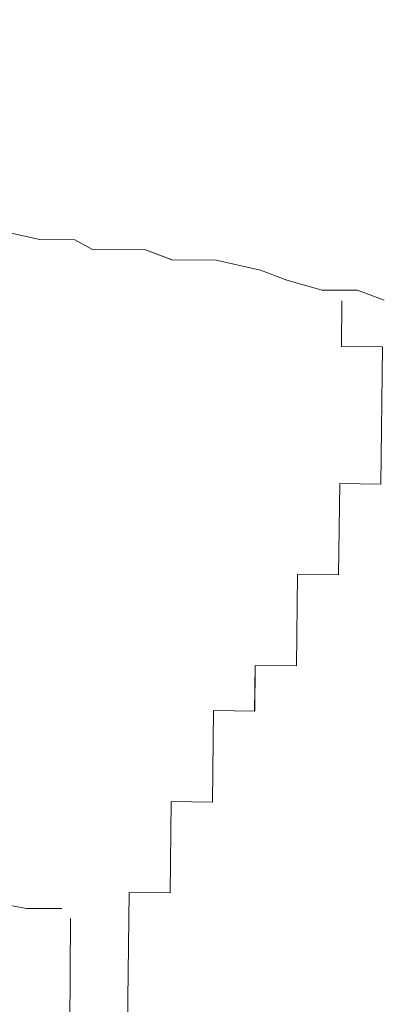
# Model space of a CAD drawing. Units: inches. Extents: x -466983 to 1020, y 324 to 318697.
# Tile 65 of 97: x 642.74 to 643.839, y 945.669 to 948.644. Entities that reach past the tile are written whole.
import ezdxf

# ---------------------------------------------------------------- set-up
doc = ezdxf.new("R2010")
doc.units = ezdxf.units.IN
doc.header["$MEASUREMENT"] = 0
doc.layers.add('A-FLOR-PATT', color=252, linetype='Continuous', lineweight=13)
doc.layers.add('A-FURN', color=8, linetype='Continuous', lineweight=18)

# ---------------------------------------------------------------- blocks, each defined once
blk = doc.blocks.new('L Shaped Sofa')
at = {"ltscale": 2}
for p, q in [((2420.3785, 737.84), (2420.403, 741.852)), ((2420.0564, 737.6965), (2420.0841, 739.9637)), ((2420.4269, 737.7856), (2420.6221, 737.7847)), ((2420.6221, 737.7847), (2420.9145, 737.7291)), ((2419.8234, 737.1954), (2419.8296, 737.6992)), ((2419.8296, 737.6992), (2420.0564, 737.6965)), ((2419.5904, 736.6944), (2419.5966, 737.1982)), ((2419.5966, 737.1982), (2419.8234, 737.1954)), ((2419.3605, 736.4452), (2419.3636, 736.6971)), ((2419.3636, 736.6971), (2419.5904, 736.6944)), ((2419.1275, 735.9442), (2419.1337, 736.448)), ((2419.1337, 736.448), (2419.3605, 736.4452)), ((2418.8945, 735.4431), (2418.9007, 735.9469)), ((2418.9007, 735.9469), (2419.1275, 735.9442)), ((2418.6584, 734.6902), (2418.6677, 735.4459)), ((2418.6677, 735.4459), (2418.8945, 735.4431)), ((2418.8853, 734.6874), (2418.6584, 734.6902)), ((2418.8822, 734.4355), (2418.8853, 734.6874)), ((2418.6497, 734.4324), (2418.7958, 734.3775)), ((2418.7958, 734.3775), (2418.9909, 734.3766)), ((2418.9909, 734.3766), (2419.1858, 734.3215)), ((2419.1858, 734.3215), (2419.3318, 734.2666)), ((2419.3318, 734.2666), (2419.5755, 734.2112)), ((2419.5755, 734.2112), (2419.8195, 734.2101)), ((2419.8195, 734.2101), (2419.9655, 734.1552)), ((2419.9655, 734.1552), (2420.2583, 734.1538)), ((2420.2583, 734.1538), (2420.3555, 734.0991)), ((2420.3555, 734.0991), (2420.5507, 734.0982)), ((2420.5507, 734.0982), (2420.7944, 734.0429))]:
    blk.add_line(p, q, dxfattribs=at)

msp = doc.modelspace()

# ---------------------------------------------------------------- hatches: boundary and pattern name
at = {"layer": 'A-FLOR-PATT', "transparency": 33554572}
h = msp.add_hatch(dxfattribs=at)
h.set_pattern_fill('ANSI37', color=256, scale=30)
h.set_pattern_definition([(45, (-1212.4137, -290.035), (-2.6516504, 2.6516504), []), (135, (-1212.4137, -290.035), (-2.6516504, -2.6516504), [])])
h.paths.add_polyline_path([(901.8057, 1075.9377), (900.6144, 1075.9377), (900.6144, 1065.3856), (899.391, 1065.3856), (898.0911, 1065.3856), (892.8356, 1058.7098, -0.258377), (892.1875, 1058.3509), (879.9848, 1058.3509, -0.20177), (879.4382, 1058.5808), (874.0812, 1065.3856), (872.7813, 1065.3856), (871.5579, 1065.3856), (871.5579, 1075.9377), (813.8057, 1075.9377), (813.8057, 1044.7922), (832.3947, 1044.7922, -0.394795), (848.6602, 1028.5356), (848.6602, 1009.9377), (901.8057, 1009.9377), (901.8057, 1015.9377), (901.3057, 1015.9377), (871.3057, 1015.9377), (871.3057, 1017.2502), (871.3344, 1017.2502, -0.401453), (901.3057, 1045.9377), (901.8057, 1045.9377)])
edge = h.paths.add_edge_path(flags=16)
edge.add_line((847.7731, 1068.9486), (847.7731, 1073.7088))
edge.add_arc((849.2269, 1073.7088), 1.4538, 90, 180, ccw=False)
edge.add_line((849.2269, 1075.1627), (864.4921, 1075.1627))
edge.add_arc((864.4921, 1073.7088), 1.4538, 0, 90, ccw=False)
edge.add_line((865.9459, 1073.7088), (865.9459, 1069.0035))
edge.add_arc((832.6447, 1068.9761), 33.3012, -20.61234, 0.04725, ccw=False)
edge.add_ellipse((856.8595, 1058.48), major_axis=(0, 10.2131), ratio=0.6859192, start_angle=100.00884, end_angle=259.99116, ccw=False)
edge.add_arc((881.0742, 1068.9761), 33.3012, 180.04725, 200.61234, ccw=False)
h.paths.add_polyline_path([(853.1456, 1066.4815), (853.1456, 1066.4534), (853.1463, 1066.4534, 0.433107), (852.9166, 1066.6849), (852.9166, 1066.4534), (853.1456, 1066.4534), (853.1456, 1066.4815), (853.088, 1066.6122, 0.697939), (852.6995, 1066.4534), (852.7003, 1066.4534), (852.7003, 1066.4815), (852.9166, 1067.0012), (852.9166, 1066.6849, -0.396254)], flags=0)
h.paths.add_polyline_path([(861.0187, 1066.4815), (861.0187, 1066.4534), (861.0194, 1066.4534, 0.416404), (860.8024, 1066.6849), (860.8024, 1066.4534), (861.0187, 1066.4534), (861.0187, 1066.4815), (860.9672, 1066.6053, 0.713344), (860.5726, 1066.4534), (860.5734, 1066.4534), (860.5734, 1066.4815), (860.8024, 1067.0012), (860.8024, 1066.6849, -0.379973)], flags=0)
edge = h.paths.add_edge_path(flags=0)
edge.add_spline(control_points=[(861.1298, 1065.7855), (861.4661, 1065.2478), (861.6134, 1065.0161), (861.9833, 1064.3736), (862.1924, 1063.9443), (862.5614, 1063.0391), (862.7212, 1062.5633), (862.9865, 1061.5781), (863.092, 1061.0689), (863.2452, 1060.031), (863.293, 1059.5025), (863.3295, 1058.4409), (863.3181, 1057.9078), (863.2366, 1056.8518), (863.1664, 1056.3289), (862.9695, 1055.308), (862.8427, 1054.8099), (862.5365, 1053.8522), (862.3571, 1053.3927), (861.9514, 1052.5249), (861.7251, 1052.1166), (861.233, 1051.3622), (860.9672, 1051.0162), (860.4048, 1050.3949), (860.1082, 1050.1197), (859.4937, 1049.6461), (859.1758, 1049.4476), (858.5276, 1049.1299), (858.1973, 1049.0107), (857.5315, 1048.8518), (857.1959, 1048.8121), (856.5249, 1048.812), (856.1894, 1048.8515), (855.5236, 1049.0101), (855.1933, 1049.1291), (854.545, 1049.4465), (854.2271, 1049.6449), (853.6124, 1050.1183), (853.3158, 1050.3933), (852.7533, 1051.0143), (852.4874, 1051.3602), (851.9952, 1052.1144), (851.7688, 1052.5225), (851.3629, 1053.3902), (851.1834, 1053.8496), (850.877, 1054.8071), (850.7501, 1055.3051), (850.553, 1056.326), (850.4827, 1056.8488), (850.401, 1057.9048), (850.3895, 1058.4379), (850.4257, 1059.4995), (850.4734, 1060.0281), (850.6265, 1061.066), (850.7318, 1061.5753), (850.9969, 1062.5605), (851.1567, 1063.0365), (851.5254, 1063.9418), (851.7345, 1064.3712), (852.1056, 1065.0164), (852.2544, 1065.2503), (852.6082, 1065.7335)], knot_values=[3.915332, 3.915332, 3.915332, 3.915332, 4.013468, 4.013468, 4.175532, 4.175532, 4.337596, 4.337596, 4.49966, 4.49966, 4.661724, 4.661724, 4.823788, 4.823788, 4.985852, 4.985852, 5.147916, 5.147916, 5.30998, 5.30998, 5.472044, 5.472044, 5.634109, 5.634109, 5.796173, 5.796173, 5.958237, 5.958237, 6.120301, 6.120301, 6.282365, 6.282365, 6.444429, 6.444429, 6.606493, 6.606493, 6.768557, 6.768557, 6.930621, 6.930621, 7.092685, 7.092685, 7.254749, 7.254749, 7.416813, 7.416813, 7.578878, 7.578878, 7.740942, 7.740942, 7.903006, 7.903006, 8.06507, 8.06507, 8.227134, 8.227134, 8.389198, 8.389198, 8.551262, 8.551262, 8.65037, 8.65037, 8.65037, 8.65037], degree=3, periodic=0)
edge.add_line((852.6421, 1065.7855), (861.1298, 1065.7855))
edge = h.paths.add_edge_path(flags=0)
edge.add_ellipse((856.8496, 1057.7432), major_axis=(0, 7.7921), ratio=0.687861, start_angle=0, end_angle=360)
h.paths.add_polyline_path([(848.8634, 1069.3891), (848.8634, 1073.9605, -0.414214), (849.9538, 1075.0508), (863.7652, 1075.0508, -0.414214), (864.8555, 1073.9605), (864.8555, 1069.3891, -0.388936), (864.5237, 1069.027, -0.043561), (849.1953, 1069.027, -0.388936)], flags=0)
h.paths.add_polyline_path([(853.1006, 1068.1122, -1), (852.6775, 1068.1122, -1)], flags=0)
edge = h.paths.add_edge_path(flags=0)
edge.add_ellipse((856.8595, 1057.3378), major_axis=(0, 2.207), ratio=0.657164, start_angle=0, end_angle=360)
h.paths.add_polyline_path([(861.0415, 1068.1122, -1), (860.6184, 1068.1122, -1)], flags=0)
edge = h.paths.add_edge_path()
edge.add_line((573.9537, 1057.3412), (573.9537, 1075.9377))
edge.add_line((573.9537, 1075.9377), (558.7308, 1075.9377))
edge.add_line((558.7308, 1075.9377), (558.7308, 1065.3856))
edge.add_line((558.7308, 1065.3856), (557.5074, 1065.3856))
edge.add_line((557.5074, 1065.3856), (556.2075, 1065.3856))
edge.add_line((556.2075, 1065.3856), (550.952, 1058.7098))
edge.add_arc((550.3039, 1059.1155), 0.7646, 270, 327.9483, ccw=False)
edge.add_line((550.3039, 1058.3509), (538.1012, 1058.3509))
edge.add_arc((538.1012, 1059.1155), 0.7646, 224.3704, 270, ccw=False)
edge.add_line((537.5546, 1058.5808), (532.1976, 1065.3856))
edge.add_line((532.1976, 1065.3856), (530.8977, 1065.3856))
edge.add_line((530.8977, 1065.3856), (529.6743, 1065.3856))
edge.add_line((529.6743, 1065.3856), (529.6743, 1075.9377))
edge.add_line((529.6743, 1075.9377), (520.8057, 1075.9377))
edge.add_line((520.8057, 1075.9377), (520.8057, 1045.9377))
edge.add_line((520.8057, 1045.9377), (521.3057, 1045.9377))
edge.add_arc((521.3057, 1015.9377), 30, 2.50749, 90, ccw=False)
edge.add_line((551.277, 1017.2502), (551.3057, 1017.2502))
edge.add_line((551.3057, 1017.2502), (551.3057, 1015.9377))
edge.add_line((551.3057, 1015.9377), (520.8057, 1015.9377))
edge.add_line((520.8057, 1015.9377), (520.8057, 1009.9377))
edge.add_line((520.8057, 1009.9377), (559.1913, 1010.4022))
edge.add_arc((559.1913, 1011.856), 1.4538, 180, 270, ccw=False)
edge.add_line((557.7375, 1011.856), (557.7375, 1016.5613))
edge.add_arc((591.0386, 1016.5888), 33.3012, 159.38766, 180.04725, ccw=False)
edge.add_ellipse((566.8239, 1027.0848), major_axis=(0, 10.2131), ratio=0.6859192, start_angle=280.00884, end_angle=439.99116, ccw=False)
edge.add_arc((542.6091, 1016.5888), 33.3012, 0.04725, 20.61234, ccw=False)
edge.add_line((575.9103, 1016.6162), (575.9103, 1011.856))
edge.add_arc((574.4565, 1011.856), 1.4538, -90, 0, ccw=False)
edge.add_line((574.4565, 1010.4022), (608.8057, 1009.9377))
edge.add_line((608.8057, 1009.9377), (608.8057, 1041.0857))
edge.add_line((608.8057, 1041.0857), (590.2179, 1041.0857))
edge.add_arc((590.775, 1057.9074), 16.8309, 181.92775, 268.10321, ccw=False)
edge = h.paths.add_edge_path()
edge.add_ellipse((494.2443, 583.6204), major_axis=(0, 10.2131), ratio=0.6859192, start_angle=280.00884, end_angle=439.99116, ccw=False)
edge.add_arc((470.0296, 573.1243), 33.3012, 0.04725, 20.61234, ccw=False)
edge.add_line((503.3307, 573.1518), (503.3307, 568.3916))
edge.add_arc((501.8769, 568.3916), 1.4538, -90, 0, ccw=False)
edge.add_line((501.8769, 566.9377), (539.8057, 566.9377))
edge.add_line((539.8057, 566.9377), (539.8057, 572.9377))
edge.add_line((539.8057, 572.9377), (539.3057, 572.9377))
edge.add_line((539.3057, 572.9377), (509.3057, 572.9377))
edge.add_line((509.3057, 572.9377), (509.3057, 574.2502))
edge.add_line((509.3057, 574.2502), (509.3344, 574.2502))
edge.add_arc((539.3057, 572.9377), 30, 90, 177.49251, ccw=False)
edge.add_line((539.3057, 602.9377), (539.8057, 602.9377))
edge.add_line((539.8057, 602.9377), (539.8057, 626.9377))
edge.add_line((539.8057, 626.9377), (531.7718, 626.9377))
edge.add_line((531.7718, 626.9377), (531.7718, 616.3856))
edge.add_line((531.7718, 616.3856), (530.5484, 616.3856))
edge.add_line((530.5484, 616.3856), (529.2485, 616.3856))
edge.add_line((529.2485, 616.3856), (523.7105, 609.3509))
edge.add_line((523.7105, 609.3509), (510.7766, 609.3509))
edge.add_line((510.7766, 609.3509), (505.2386, 616.3856))
edge.add_line((505.2386, 616.3856), (503.9387, 616.3856))
edge.add_line((503.9387, 616.3856), (502.7153, 616.3856))
edge.add_line((502.7153, 616.3856), (502.7153, 626.9377))
edge.add_line((502.7153, 626.9377), (481.6983, 626.9377))
edge.add_line((481.6983, 626.9377), (481.6983, 610.995))
edge.add_arc((467.2703, 611.4728), 14.4359, 271.92775, 358.10321, ccw=False)
edge.add_line((467.7559, 597.0451), (451.8057, 597.0451))
edge.add_line((451.8057, 597.0451), (451.8057, 584.4035))
edge.add_line((451.8057, 584.4035), (451.8057, 566.9377))
edge.add_line((451.8057, 566.9377), (486.6117, 566.9377))
edge.add_arc((486.6117, 568.3916), 1.4538, 180, 270, ccw=False)
edge.add_line((485.1579, 568.3916), (485.1579, 573.0969))
edge.add_arc((518.4591, 573.1243), 33.3012, 159.38766, 180.04725, ccw=False)
h.paths.add_polyline_path([(836.2609, 1020.7328), (879.8898, 1020.7328), (879.8898, 1039.3902), (836.2609, 1039.3902)], flags=25)
h.paths.add_polyline_path([(549.9851, 1036.7492), (593.614, 1036.7492), (593.614, 1055.4065), (549.9851, 1055.4065)], flags=24)
h.paths.add_polyline_path([(475.123, 595.5959), (518.752, 595.5959), (518.752, 614.2532), (475.123, 614.2532)], flags=24)
h = msp.add_hatch(dxfattribs=at)
h.set_pattern_fill('ANSI37', color=256, scale=20)
h.set_pattern_definition([(45, (-1212.4137, -290.035), (-1.767767, 1.767767), []), (135, (-1212.4137, -290.035), (-1.767767, -1.767767), [])])
h.paths.add_polyline_path([(809.8057, 870.9377), (809.8057, 888.1519), (806.9985, 888.1519), (802.6624, 888.1519), (789.3832, 888.1519), (786.2846, 888.1519, -0.414214), (785.4991, 888.9374), (785.4991, 900.1959), (785.4991, 908.4696, -0.414214), (786.8082, 909.7787, -0.414214), (785.4991, 911.0878), (785.4991, 929.1015, -0.414214), (786.8082, 930.4106, -0.414214), (785.4991, 931.7197), (785.4991, 931.9039, -0.414214), (784.19, 930.5948), (766.7223, 930.5948, -0.412359), (765.4132, 931.8956, -0.413741), (764.1145, 930.5782), (744.5781, 930.422, -0.416556), (743.7864, 931.2075), (743.7864, 933.5153), (742.2154, 933.5153), (742.2154, 952.024, -0.001344), (743.7864, 952.1998), (743.7864, 953.9377), (678.5915, 953.9377), (678.5915, 951.1305), (678.5915, 946.7945), (678.5915, 933.5153), (678.5915, 930.4166, -0.414214), (677.806, 929.6312), (666.5475, 929.6312), (658.2738, 929.6312, -0.414214), (656.9647, 930.9403, -0.414214), (655.6556, 929.6312), (637.6419, 929.6312, -0.414214), (636.3328, 930.9403, -0.414214), (635.0237, 929.6312), (634.8395, 929.6312, -0.414214), (636.1486, 928.322), (636.1486, 910.8544, -0.412359), (634.8478, 909.5452, -0.413741), (636.1653, 908.2466), (636.3214, 888.7102, -0.416556), (635.5359, 887.9184), (633.2281, 887.9184), (633.2281, 886.3475), (614.7194, 886.3475, -0.001344), (614.5436, 887.9184), (612.8057, 887.9184), (612.8057, 834.9377), (612.8057, 752.9377), (612.8057, 748.9377), (612.8057, 697.9377), (654.8057, 697.9377), (654.8057, 701.9377), (715.8057, 701.9377), (715.8057, 737.4353), (774.2918, 737.4353), (774.2918, 795.9377), (809.8057, 795.9377)])
h.paths.add_polyline_path([(679.2761, 849.5757, 0.102523), (682.1475, 849.2608, -0.080461), (694.5428, 849.7725, -0.283899), (694.4822, 849.0082, 0.136605), (694.4068, 848.8103, -0.030441), (694.5428, 846.8929), (694.5428, 842.6198), (694.5428, 838.3466, -0.028219), (694.4246, 836.5684), (694.425, 836.5684, 0.196187), (694.4456, 836.2708, -0.302897), (694.5428, 835.467, -0.080461), (682.1475, 835.9787, 0.102523), (679.2761, 835.6638, -0.58611), (678.6457, 836.0169), (678.6457, 849.2227, -0.58611)], flags=16)
h.paths.add_polyline_path([(679.5173, 848.6515, 0.699597), (679.476, 848.6342, 1.20716), (679.1935, 848.7422, 0.010621)], flags=0)
h.paths.add_polyline_path([(679.4923, 836.5608, -0.013798), (679.9178, 836.6594, -0.071703), (682.8533, 837.1434, -0.165743), (682.1665, 839.1006), (682.1665, 842.6094), (682.1665, 846.0603, -0.240616), (683.4733, 848.6767, -0.068263), (693.9295, 849.0082), (693.7875, 848.7083), (693.7875, 849.0228, 0.067332), (683.4733, 848.6767, 0.240616), (682.1665, 846.0603), (682.1665, 842.6094), (682.1665, 839.1006, 0.23459), (683.461, 836.5513, 0.068093), (693.7875, 836.1955), (693.7875, 836.5104), (693.9296, 836.2102, -0.077215), (682.2421, 836.7815, 0.086627), (679.5283, 836.5701, -0.628402), (679.5029, 836.5735), (679.5029, 836.6071, 0.910458)], flags=0)
h.paths.add_polyline_path([(679.476, 848.6364), (679.2069, 848.647), (679.2069, 836.5718, 0.913566), (679.3645, 836.5861), (679.476, 836.5824)], flags=0)
h.paths.add_polyline_path([(679.2761, 829.8604, 0.102523), (682.1475, 829.5455, -0.080461), (694.5428, 830.0572, -0.283899), (694.4822, 829.2929, 0.136605), (694.4068, 829.095, -0.030441), (694.5428, 827.1776), (694.5428, 822.9045), (694.5428, 818.6314, -0.028219), (694.4246, 816.8531), (694.425, 816.8532, 0.196187), (694.4456, 816.5555, -0.302897), (694.5428, 815.7517, -0.080461), (682.1475, 816.2635, 0.102523), (679.2761, 815.9485, -0.58611), (678.6457, 816.3016), (678.6457, 829.5074, -0.58611)], flags=16)
h.paths.add_polyline_path([(679.5173, 828.9362, 0.699597), (679.476, 828.9189, 1.20716), (679.1935, 829.0269, 0.010621)], flags=0)
h.paths.add_polyline_path([(679.4923, 816.8456, -0.013798), (679.9178, 816.9441, -0.071703), (682.8533, 817.4281, -0.165743), (682.1665, 819.3853), (682.1665, 822.8941), (682.1665, 826.345, -0.240616), (683.4733, 828.9614, -0.068263), (693.9295, 829.2929), (693.7875, 828.9931), (693.7875, 829.3076, 0.067332), (683.4733, 828.9614, 0.240616), (682.1665, 826.345), (682.1665, 822.8941), (682.1665, 819.3853, 0.23459), (683.461, 816.836, 0.068093), (693.7875, 816.4802), (693.7875, 816.7952), (693.9296, 816.4949, -0.077215), (682.2421, 817.0662, 0.086627), (679.5283, 816.8549, -0.628402), (679.5029, 816.8582), (679.5029, 816.8918, 0.910458)], flags=0)
h.paths.add_polyline_path([(679.476, 828.9211), (679.2069, 828.9317), (679.2069, 816.8565, 0.913566), (679.3645, 816.8708), (679.476, 816.8671)], flags=0)
h.paths.add_polyline_path([(679.2761, 810.1451, 0.102523), (682.1475, 809.8302, -0.080461), (694.5428, 810.342, -0.3023), (694.4466, 809.5394, 0.10023), (694.4058, 809.3878, -0.03057), (694.5428, 807.4623), (694.5428, 803.1892), (694.5428, 798.9161, -0.03057), (694.4058, 796.9906, 0.10023), (694.4466, 796.839, -0.3023), (694.5428, 796.0365, -0.080461), (682.1475, 796.5482, 0.102523), (679.2761, 796.2333, -0.58611), (678.6457, 796.5863), (678.6457, 809.7921, -0.58611)], flags=16)
h.paths.add_polyline_path([(679.5173, 809.2417, 0.699597), (679.476, 809.2244, 1.20716), (679.1935, 809.3324, 0.010621)], flags=0)
h.paths.add_polyline_path([(679.4923, 797.151, -0.013798), (679.9178, 797.2496, -0.071703), (682.8533, 797.7336, -0.165743), (682.1665, 799.6908), (682.1665, 803.1996), (682.1665, 806.6505, -0.239349), (683.461, 809.2577, -0.072465), (694.4468, 809.5405, 0.197932), (694.425, 809.2405), (693.7875, 809.2985), (693.7875, 809.6135, 0.068093), (683.461, 809.2577, 0.239349), (682.1665, 806.6505), (682.1665, 803.1996), (682.1665, 799.6908, 0.235854), (683.4733, 797.1323, 0.067332), (693.7875, 796.7861), (693.7875, 797.1006), (694.425, 797.1586, 0.197932), (694.4468, 796.8586, -0.080419), (682.1557, 797.3795, 0.083867), (679.5283, 797.1603, -0.628402), (679.5029, 797.1637), (679.5029, 797.1973, 0.910458)], flags=0)
h.paths.add_polyline_path([(679.2069, 809.2372), (679.2069, 797.162, 0.913566), (679.3645, 797.1763), (679.476, 797.1726), (679.476, 809.2266)], flags=0)
h.paths.add_polyline_path([(695.3643, 853.2989), (728.2231, 853.2989), (728.2231, 771.1519), (695.3643, 771.1519)], flags=16)
h.paths.add_polyline_path([(696.0215, 852.6417), (727.5659, 852.6417), (727.5659, 771.809), (696.0215, 771.809)], flags=0)
h.paths.add_polyline_path([(679.2761, 788.7869, 0.102523), (682.1475, 788.472, -0.080461), (694.5428, 788.9837, -0.3023), (694.4466, 788.1812, 0.10023), (694.4058, 788.0296, -0.03057), (694.5428, 786.1041), (694.5428, 781.831), (694.5428, 777.5578, -0.03057), (694.4058, 775.6323, 0.10023), (694.4466, 775.4808, -0.3023), (694.5428, 774.6782, -0.080461), (682.1475, 775.19, 0.102523), (679.2761, 774.875, -0.58611), (678.6457, 775.2281), (678.6457, 788.4339, -0.58611)], flags=16)
h.paths.add_polyline_path([(679.5173, 787.8834, 0.699597), (679.476, 787.8662, 1.20716), (679.1935, 787.9742, 0.010621)], flags=0)
h.paths.add_polyline_path([(679.4923, 775.7928, -0.013798), (679.9178, 775.8914, -0.071703), (682.8533, 776.3753, -0.165743), (682.1665, 778.3325), (682.1665, 781.8414), (682.1665, 785.2922, -0.239349), (683.461, 787.8995, -0.072465), (694.4468, 788.1823, 0.197932), (694.425, 787.8823), (693.7875, 787.9403), (693.7875, 788.2553, 0.068093), (683.461, 787.8995, 0.239349), (682.1665, 785.2922), (682.1665, 781.8414), (682.1665, 778.3325, 0.235854), (683.4733, 775.7741, 0.067332), (693.7875, 775.4279), (693.7875, 775.7424), (694.425, 775.8004, 0.197932), (694.4468, 775.5004, -0.080419), (682.1557, 776.0212, 0.083867), (679.5283, 775.8021, -0.628402), (679.5029, 775.8054), (679.5029, 775.8391, 0.910458)], flags=0)
h.paths.add_polyline_path([(679.2069, 787.8789), (679.2069, 775.8038, 0.913566), (679.3645, 775.818), (679.476, 775.8144), (679.476, 787.8684)], flags=0)
h.paths.add_polyline_path([(704.641, 854.1204, -0.080461), (705.1527, 866.5157, 0.102523), (704.8378, 869.3871, -0.58611), (705.1908, 870.0174), (718.3966, 870.0174, -0.58611), (718.7496, 869.3871, 0.102523), (718.4347, 866.5157, -0.080461), (718.9465, 854.1204, -0.3023), (718.1439, 854.2166, 0.10023), (717.9924, 854.2574, -0.03057), (716.0668, 854.1204), (711.7937, 854.1204), (707.5206, 854.1204, -0.03057), (705.5951, 854.2574, 0.10023), (705.4435, 854.2166, -0.3023)], flags=16)
h.paths.add_polyline_path([(717.8462, 869.1459, 0.699597), (717.8289, 869.1872, 1.20716), (717.9369, 869.4697, 0.010621)], flags=0)
h.paths.add_polyline_path([(705.4631, 854.2164, -0.080419), (705.984, 866.5074, 0.083867), (705.7648, 869.1349, -0.628402), (705.7682, 869.1603), (705.8018, 869.1603, 0.910458), (705.7555, 869.1709, -0.013798), (705.8541, 868.7454, -0.071703), (706.3381, 865.8099, -0.165743), (708.2953, 866.4967), (711.8041, 866.4967), (715.255, 866.4967, -0.239349), (717.8622, 865.2022, -0.072465), (718.145, 854.2164, 0.197932), (717.845, 854.2382), (717.903, 854.8757), (718.218, 854.8757, 0.068093), (717.8622, 865.2022, 0.239349), (715.255, 866.4967), (711.8041, 866.4967), (708.2953, 866.4967, 0.235854), (705.7368, 865.1898, 0.067332), (705.3906, 854.8757), (705.7051, 854.8757), (705.7631, 854.2382, 0.197932)], flags=16)
h.paths.add_polyline_path([(705.7665, 869.4563, 0.913566), (705.7808, 869.2987), (705.7771, 869.1872), (717.8311, 869.1872), (717.8417, 869.4563)], flags=0)
h.paths.add_polyline_path([(729.0446, 842.6198), (729.0446, 846.8929, -0.03057), (729.1817, 848.8184, 0.10023), (729.1408, 848.9699, -0.3023), (729.0446, 849.7725, -0.080461), (741.4399, 849.2608, 0.102523), (744.3113, 849.5757, -0.58611), (744.9417, 849.2227), (744.9417, 836.0169, -0.58611), (744.3113, 835.6638, 0.102523), (741.4399, 835.9787, -0.080461), (729.0446, 835.467, -0.3023), (729.1408, 836.2696, 0.10023), (729.1817, 836.4211, -0.03057), (729.0446, 838.3466)], flags=16)
h.paths.add_polyline_path([(744.1115, 836.5846, 1.20716), (744.3939, 836.4766, 0.010621), (744.0701, 836.5673, 0.699597)], flags=0)
h.paths.add_polyline_path([(729.1407, 836.2684, 0.197932), (729.1624, 836.5684), (729.7999, 836.5104), (729.7999, 836.1955, 0.068093), (740.1264, 836.5513, 0.239349), (741.4209, 839.1585), (741.4209, 842.6094), (741.4209, 846.1182, 0.235854), (740.1141, 848.6767, 0.067332), (729.7999, 849.0228), (729.7999, 848.7083), (729.1624, 848.6503, 0.197932), (729.1407, 848.9504, -0.080419), (741.4317, 848.4295, 0.083867), (744.0591, 848.6486, -0.628402), (744.0845, 848.6453), (744.0845, 848.6117, 0.910458), (744.0951, 848.6579, -0.013798), (743.6696, 848.5594, -0.071703), (740.7341, 848.0754, -0.165743), (741.4209, 846.1182), (741.4209, 842.6094), (741.4209, 839.1585, -0.239349), (740.1264, 836.5513, -0.072465)], flags=0)
h.paths.add_polyline_path([(729.0446, 830.0572, -0.080461), (741.4399, 829.5455, 0.102523), (744.3113, 829.8604, -0.58611), (744.9417, 829.5074), (744.9417, 816.3016, -0.58611), (744.3113, 815.9485, 0.102523), (741.4399, 816.2635, -0.080461), (729.0446, 815.7517, -0.3023), (729.1408, 816.5543, 0.10023), (729.1817, 816.7058, -0.03057), (729.0446, 818.6314), (729.0446, 822.9045), (729.0446, 827.1776, -0.03057), (729.1817, 829.1031, 0.10023), (729.1408, 829.2547, -0.3023)], flags=16)
h.paths.add_polyline_path([(744.1115, 816.8693, 1.20716), (744.3939, 816.7613, 0.010621), (744.0701, 816.852, 0.699597)], flags=0)
h.paths.add_polyline_path([(729.1407, 829.2351, -0.080419), (741.4317, 828.7142, 0.083867), (744.0591, 828.9334, -0.628402), (744.0845, 828.93), (744.0845, 828.8964, 0.910458), (744.0951, 828.9427, -0.013798), (743.6696, 828.8441, -0.071703), (740.7341, 828.3601, -0.165743), (741.4209, 826.4029), (741.4209, 822.8941), (741.4209, 819.4432, -0.239349), (740.1264, 816.836, -0.072465), (729.1407, 816.5531, 0.197932), (729.1624, 816.8532), (729.7999, 816.7952), (729.7999, 816.4802, 0.068093), (740.1264, 816.836, 0.239349), (741.4209, 819.4432), (741.4209, 822.8941), (741.4209, 826.4029, 0.235854), (740.1141, 828.9614, 0.067332), (729.7999, 829.3076), (729.7999, 828.9931), (729.1624, 828.9351, 0.197932)], flags=16)
h.paths.add_polyline_path([(729.0446, 810.342, -0.080461), (741.4399, 809.8302, 0.102523), (744.3113, 810.1451, -0.58611), (744.9417, 809.7921), (744.9417, 796.5863, -0.58611), (744.3113, 796.2333, 0.102523), (741.4399, 796.5482, -0.080461), (729.0446, 796.0365, -0.283899), (729.1052, 796.8007, 0.136605), (729.1806, 796.9987, -0.030441), (729.0446, 798.9161), (729.0446, 803.1892), (729.0446, 807.4623, -0.028219), (729.1628, 809.2406), (729.1624, 809.2405, 0.196187), (729.1418, 809.5382, -0.302897)], flags=16)
h.paths.add_polyline_path([(744.1115, 797.1748, 1.20716), (744.3939, 797.0668, 0.010621), (744.0701, 797.1575, 0.699597)], flags=0)
h.paths.add_polyline_path([(741.3453, 809.0275, 0.086627), (744.0591, 809.2388, -0.628402), (744.0845, 809.2355), (744.0845, 809.2019, 0.910458), (744.0951, 809.2481, -0.013798), (743.6696, 809.1496, -0.071703), (740.7341, 808.6656, -0.165743), (741.4209, 806.7084), (741.4209, 803.1996), (741.4209, 799.7487, -0.240616), (740.1141, 797.1323, -0.068263), (729.658, 796.8008), (729.7999, 797.1006), (729.7999, 796.7861, 0.067332), (740.1141, 797.1323, 0.240616), (741.4209, 799.7487), (741.4209, 803.1996), (741.4209, 806.7084, 0.23459), (740.1264, 809.2577, 0.068093), (729.7999, 809.6135), (729.7999, 809.2985), (729.6578, 809.5988, -0.077215)], flags=0)
h.paths.add_polyline_path([(704.641, 770.3304, -0.283899), (705.4053, 770.2697, 0.136605), (705.6032, 770.1944, -0.030441), (707.5206, 770.3304), (711.7937, 770.3304), (716.0668, 770.3304, -0.028219), (717.8451, 770.2122), (717.845, 770.2126, 0.196187), (718.1427, 770.2331, -0.302897), (718.9465, 770.3304, -0.080461), (718.4347, 757.9351, 0.102523), (718.7496, 755.0637, -0.58611), (718.3966, 754.4333), (705.1908, 754.4333, -0.58611), (704.8378, 755.0637, 0.102523), (705.1527, 757.9351, -0.080461)], flags=16)
h.paths.add_polyline_path([(705.762, 755.3048, 0.699597), (705.7793, 755.2635, 1.20716), (705.6713, 754.9811, 0.010621)], flags=0)
h.paths.add_polyline_path([(705.4053, 769.717), (705.7051, 769.5751), (705.3906, 769.5751, 0.067332), (705.7368, 759.2609, 0.240616), (708.3532, 757.954), (711.8041, 757.954), (715.3129, 757.954, 0.23459), (717.8622, 759.2485, 0.068093), (718.218, 769.5751), (717.903, 769.5751), (718.2033, 769.7172, -0.077215), (717.632, 758.0297, 0.086627), (717.8433, 755.3159, -0.628402), (717.84, 755.2904), (717.8064, 755.2904, 0.910458), (717.8526, 755.2799, -0.013798), (717.7541, 755.7053, -0.071703), (717.2701, 758.6409, -0.165743), (715.3129, 757.954), (711.8041, 757.954), (708.3532, 757.954, -0.240616), (705.7368, 759.2609, -0.068263)], flags=0)
h.paths.add_polyline_path([(729.0446, 788.9837, -0.080461), (741.4399, 788.472, 0.102523), (744.3113, 788.7869, -0.58611), (744.9417, 788.4339), (744.9417, 775.2281, -0.58611), (744.3113, 774.875, 0.102523), (741.4399, 775.19, -0.080461), (729.0446, 774.6782, -0.283899), (729.1052, 775.4425, 0.136605), (729.1806, 775.6405, -0.030441), (729.0446, 777.5578), (729.0446, 781.831), (729.0446, 786.1041, -0.028219), (729.1628, 787.8823), (729.1624, 787.8823, 0.196187), (729.1418, 788.1799, -0.302897)], flags=16)
h.paths.add_polyline_path([(744.1115, 775.8165, 1.20716), (744.3939, 775.7086, 0.010621), (744.0701, 775.7993, 0.699597)], flags=0)
h.paths.add_polyline_path([(741.3453, 787.6692, 0.086627), (744.0591, 787.8806, -0.628402), (744.0845, 787.8773), (744.0845, 787.8437, 0.910458), (744.0951, 787.8899, -0.013798), (743.6696, 787.7913, -0.071703), (740.7341, 787.3074, -0.165743), (741.4209, 785.3502), (741.4209, 781.8414), (741.4209, 778.3905, -0.240616), (740.1141, 775.7741, -0.068263), (729.658, 775.4425), (729.7999, 775.7424), (729.7999, 775.4279, 0.067332), (740.1141, 775.7741, 0.240616), (741.4209, 778.3905), (741.4209, 781.8414), (741.4209, 785.3502, 0.23459), (740.1264, 787.8995, 0.068093), (729.7999, 788.2553), (729.7999, 787.9403), (729.6578, 788.2405, -0.077215)], flags=0)
h.paths.add_polyline_path([(744.1115, 848.6364), (744.1115, 836.5824), (744.3805, 836.5718), (744.3805, 848.647, 0.913566), (744.2229, 848.6327)], flags=0)
h.paths.add_polyline_path([(744.2229, 828.9174), (744.1115, 828.9211), (744.1115, 816.8671), (744.3805, 816.8565), (744.3805, 828.9317, 0.913566)], flags=0)
h.paths.add_polyline_path([(717.8311, 755.2635), (705.7771, 755.2635), (705.7665, 754.9945), (717.8417, 754.9945, 0.913566), (717.8274, 755.1521)], flags=0)
h.paths.add_polyline_path([(744.2229, 809.2229), (744.1115, 809.2266), (744.1115, 797.1726), (744.3805, 797.162), (744.3805, 809.2372, 0.913566)], flags=0)
h.paths.add_polyline_path([(744.1115, 787.8684), (744.1115, 775.8144), (744.3805, 775.8038), (744.3805, 787.8789, 0.913566), (744.2229, 787.8647)], flags=0)
h.paths.add_polyline_path([(678.8774, 877.1228), (737.6127, 877.1228), (737.6127, 899.5116), (678.8774, 899.5116)], flags=24)

# ---------------------------------------------------------------- linework, layer by layer
at = {"layer": 'A-FURN', "ltscale": 2}
for p, q in [((642.7997, 947.9793), (642.6661, 948.0096)), ((642.7997, 947.9793), (642.6661, 948.0096)), ((642.7997, 947.9793), (642.6661, 948.0096)), ((642.7997, 947.9793), (642.6661, 948.0096)), ((642.7997, 947.9793), (642.6661, 948.0096)), ((642.7997, 947.9793), (642.6661, 948.0096)), ((642.9067, 947.9788), (642.7997, 947.9793)), ((642.9067, 947.9788), (642.7997, 947.9793)), ((642.9067, 947.9788), (642.7997, 947.9793)), ((642.9067, 947.9788), (642.7997, 947.9793)), ((642.9067, 947.9788), (642.7997, 947.9793)), ((642.9067, 947.9788), (642.7997, 947.9793)), ((642.96, 947.9488), (642.9067, 947.9788)), ((642.96, 947.9488), (642.9067, 947.9788)), ((642.96, 947.9488), (642.9067, 947.9788)), ((642.96, 947.9488), (642.9067, 947.9788)), ((642.96, 947.9488), (642.9067, 947.9788)), ((642.96, 947.9488), (642.9067, 947.9788)), ((643.1205, 947.9481), (642.96, 947.9488)), ((643.1205, 947.9481), (642.96, 947.9488)), ((643.1205, 947.9481), (642.96, 947.9488)), ((643.1205, 947.9481), (642.96, 947.9488)), ((643.1205, 947.9481), (642.96, 947.9488)), ((643.1205, 947.9481), (642.96, 947.9488)), ((643.2006, 947.918), (643.1205, 947.9481)), ((643.2006, 947.918), (643.1205, 947.9481)), ((643.2006, 947.918), (643.1205, 947.9481)), ((643.2006, 947.918), (643.1205, 947.9481)), ((643.2006, 947.918), (643.1205, 947.9481)), ((643.2006, 947.918), (643.1205, 947.9481)), ((643.3343, 947.9173), (643.2006, 947.918)), ((643.3343, 947.9173), (643.2006, 947.918)), ((643.3343, 947.9173), (643.2006, 947.918)), ((643.3343, 947.9173), (643.2006, 947.918)), ((643.3343, 947.9173), (643.2006, 947.918)), ((643.3343, 947.9173), (643.2006, 947.918)), ((643.4679, 947.887), (643.3343, 947.9173)), ((643.4679, 947.887), (643.3343, 947.9173)), ((643.4679, 947.887), (643.3343, 947.9173)), ((643.4679, 947.887), (643.3343, 947.9173)), ((643.4679, 947.887), (643.3343, 947.9173)), ((643.4679, 947.887), (643.3343, 947.9173)), ((643.548, 947.8569), (643.4679, 947.887)), ((643.548, 947.8569), (643.4679, 947.887)), ((643.548, 947.8569), (643.4679, 947.887)), ((643.548, 947.8569), (643.4679, 947.887)), ((643.548, 947.8569), (643.4679, 947.887)), ((643.548, 947.8569), (643.4679, 947.887)), ((643.6548, 947.8267), (643.548, 947.8569)), ((643.6548, 947.8267), (643.548, 947.8569)), ((643.6548, 947.8267), (643.548, 947.8569)), ((643.6548, 947.8267), (643.548, 947.8569)), ((643.6548, 947.8267), (643.548, 947.8569)), ((643.6548, 947.8267), (643.548, 947.8569)), ((643.7618, 947.8262), (643.6548, 947.8267)), ((643.7618, 947.8262), (643.6548, 947.8267)), ((643.7618, 947.8262), (643.6548, 947.8267)), ((643.7618, 947.8262), (643.6548, 947.8267)), ((643.7618, 947.8262), (643.6548, 947.8267)), ((643.7618, 947.8262), (643.6548, 947.8267)), ((643.8418, 947.7961), (643.7618, 947.8262)), ((643.8418, 947.7961), (643.7618, 947.8262)), ((643.8418, 947.7961), (643.7618, 947.8262)), ((643.8418, 947.7961), (643.7618, 947.8262)), ((643.8418, 947.7961), (643.7618, 947.8262)), ((643.8418, 947.7961), (643.7618, 947.8262)), ((643.7144, 947.7944), (643.7127, 947.6563)), ((643.7144, 947.7944), (643.7127, 947.6563)), ((643.7144, 947.7944), (643.7127, 947.6563)), ((643.7144, 947.7944), (643.7127, 947.6563)), ((643.7144, 947.7944), (643.7127, 947.6563)), ((643.7144, 947.7944), (643.7127, 947.6563)), ((643.7127, 947.6563), (643.8371, 947.6548)), ((643.7127, 947.6563), (643.8371, 947.6548)), ((643.7127, 947.6563), (643.8371, 947.6548)), ((643.7127, 947.6563), (643.8371, 947.6548)), ((643.7127, 947.6563), (643.8371, 947.6548)), ((643.7127, 947.6563), (643.8371, 947.6548)), ((643.8371, 947.6548), (643.832, 947.2405)), ((643.8371, 947.6548), (643.832, 947.2405)), ((643.8371, 947.6548), (643.832, 947.2405)), ((643.8371, 947.6548), (643.832, 947.2405)), ((643.8371, 947.6548), (643.832, 947.2405)), ((643.8371, 947.6548), (643.832, 947.2405)), ((643.7076, 947.242), (643.7043, 946.9658)), ((643.7076, 947.242), (643.7043, 946.9658)), ((643.7076, 947.242), (643.7043, 946.9658)), ((643.7076, 947.242), (643.7043, 946.9658)), ((643.7076, 947.242), (643.7043, 946.9658)), ((643.7076, 947.242), (643.7043, 946.9658)), ((643.832, 947.2405), (643.7076, 947.242)), ((643.832, 947.2405), (643.7076, 947.242)), ((643.832, 947.2405), (643.7076, 947.242)), ((643.832, 947.2405), (643.7076, 947.242)), ((643.832, 947.2405), (643.7076, 947.242)), ((643.832, 947.2405), (643.7076, 947.242)), ((643.5799, 946.9673), (643.5765, 946.6911)), ((643.5799, 946.9673), (643.5765, 946.6911)), ((643.5799, 946.9673), (643.5765, 946.6911)), ((643.5799, 946.9673), (643.5765, 946.6911)), ((643.5799, 946.9673), (643.5765, 946.6911)), ((643.5799, 946.9673), (643.5765, 946.6911)), ((643.7043, 946.9658), (643.5799, 946.9673)), ((643.7043, 946.9658), (643.5799, 946.9673)), ((643.7043, 946.9658), (643.5799, 946.9673)), ((643.7043, 946.9658), (643.5799, 946.9673)), ((643.7043, 946.9658), (643.5799, 946.9673)), ((643.7043, 946.9658), (643.5799, 946.9673)), ((643.4522, 946.6926), (643.4505, 946.5545)), ((643.4522, 946.6926), (643.4505, 946.5545)), ((643.4522, 946.6926), (643.4505, 946.5545)), ((643.4522, 946.6926), (643.4505, 946.5545)), ((643.4522, 946.6926), (643.4505, 946.5545)), ((643.4522, 946.6926), (643.4505, 946.5545)), ((643.5765, 946.6911), (643.4522, 946.6926)), ((643.5765, 946.6911), (643.4522, 946.6926)), ((643.5765, 946.6911), (643.4522, 946.6926)), ((643.5765, 946.6911), (643.4522, 946.6926)), ((643.5765, 946.6911), (643.4522, 946.6926)), ((643.5765, 946.6911), (643.4522, 946.6926)), ((643.3261, 946.556), (643.3228, 946.2798)), ((643.3261, 946.556), (643.3228, 946.2798)), ((643.3261, 946.556), (643.3228, 946.2798)), ((643.3261, 946.556), (643.3228, 946.2798)), ((643.3261, 946.556), (643.3228, 946.2798)), ((643.3261, 946.556), (643.3228, 946.2798)), ((643.4505, 946.5545), (643.3261, 946.556)), ((643.4505, 946.5545), (643.3261, 946.556)), ((643.4505, 946.5545), (643.3261, 946.556)), ((643.4505, 946.5545), (643.3261, 946.556)), ((643.4505, 946.5545), (643.3261, 946.556)), ((643.4505, 946.5545), (643.3261, 946.556)), ((643.1984, 946.2814), (643.195, 946.0052)), ((643.1984, 946.2814), (643.195, 946.0052)), ((643.1984, 946.2814), (643.195, 946.0052)), ((643.1984, 946.2814), (643.195, 946.0052)), ((643.1984, 946.2814), (643.195, 946.0052)), ((643.1984, 946.2814), (643.195, 946.0052)), ((643.3228, 946.2798), (643.1984, 946.2814)), ((643.3228, 946.2798), (643.1984, 946.2814)), ((643.3228, 946.2798), (643.1984, 946.2814)), ((643.3228, 946.2798), (643.1984, 946.2814)), ((643.3228, 946.2798), (643.1984, 946.2814)), ((643.3228, 946.2798), (643.1984, 946.2814)), ((642.7606, 945.9583), (642.6002, 945.9888)), ((642.7606, 945.9583), (642.6002, 945.9888)), ((642.7606, 945.9583), (642.6002, 945.9888)), ((642.7606, 945.9583), (642.6002, 945.9888)), ((642.7606, 945.9583), (642.6002, 945.9888)), ((642.7606, 945.9583), (642.6002, 945.9888)), ((643.0707, 946.0067), (643.0555, 944.7638)), ((643.0707, 946.0067), (643.0555, 944.7638)), ((643.0707, 946.0067), (643.0555, 944.7638)), ((643.0707, 946.0067), (643.0555, 944.7638)), ((643.0707, 946.0067), (643.0555, 944.7638)), ((643.0707, 946.0067), (643.0555, 944.7638)), ((643.195, 946.0052), (643.0707, 946.0067)), ((643.195, 946.0052), (643.0707, 946.0067)), ((643.195, 946.0052), (643.0707, 946.0067)), ((643.195, 946.0052), (643.0707, 946.0067)), ((643.195, 946.0052), (643.0707, 946.0067)), ((643.195, 946.0052), (643.0707, 946.0067)), ((642.8676, 945.9578), (642.7606, 945.9583)), ((642.8676, 945.9578), (642.7606, 945.9583)), ((642.8676, 945.9578), (642.7606, 945.9583)), ((642.8676, 945.9578), (642.7606, 945.9583)), ((642.8676, 945.9578), (642.7606, 945.9583)), ((642.8676, 945.9578), (642.7606, 945.9583)), ((642.8941, 945.928), (642.8807, 943.7285)), ((642.8941, 945.928), (642.8807, 943.7285)), ((642.8941, 945.928), (642.8807, 943.7285)), ((642.8941, 945.928), (642.8807, 943.7285)), ((642.8941, 945.928), (642.8807, 943.7285)), ((642.8941, 945.928), (642.8807, 943.7285))]:
    msp.add_line(p, q, dxfattribs=at)

# ---------------------------------------------------------------- block references
at = {"layer": 'A-FURN', "xscale": 0.5482153745360612, "yscale": 0.5482153745360612, "zscale": 0.5482153745360612, "rotation": 180}
msp.add_blockref('L Shaped Sofa', (1969.7828, 1350.4232), dxfattribs=at)

doc.saveas('drawing.dxf')
